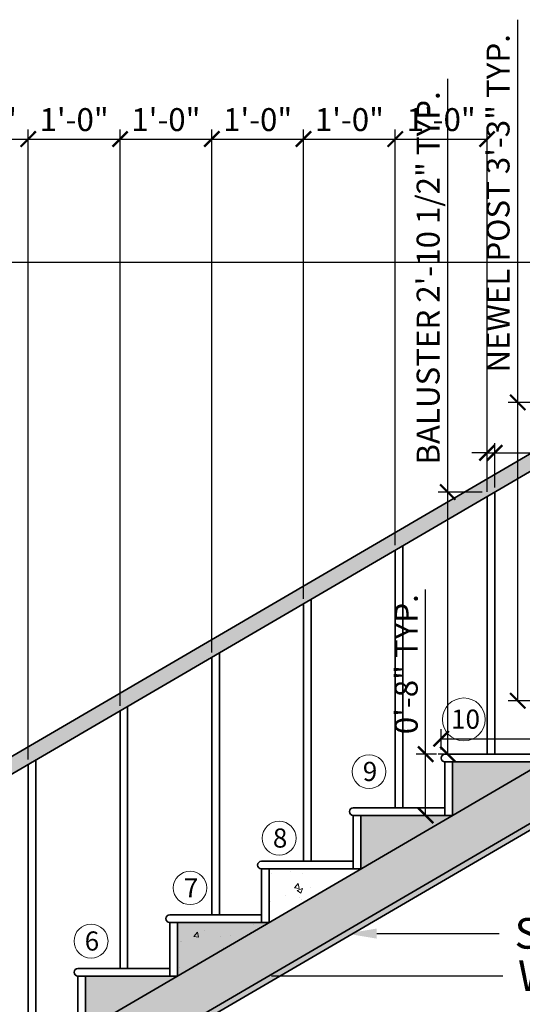
# Model space of a CAD drawing. Units: inches. Extents: x 2205 to 2524, y 4609 to 4803.
# Tile 3 of 5: x 2311 to 2377, y 4674 to 4803. Entities that reach past the tile are written whole.
import ezdxf
from ezdxf import colors
from ezdxf.entities.mleader import LeaderData, LeaderLine
from ezdxf.math import Vec2, Vec3

# ---------------------------------------------------------------- set-up
doc = ezdxf.new("R2010")
doc.units = ezdxf.units.IN
for name, color, linetype, lineweight in [('A-ANNO-DIMS', 2, 'Continuous', 18), ('A-ANNO-SYMB', 3, 'Continuous', 18), ('A-ANNO-TEXT', 7, 'Continuous', 18), ('A-FLOR-STRS', 7, 'Continuous', 35), ('A-SECT-PATT', 252, 'Continuous', 13)]:
    doc.layers.add(name, color=color, linetype=linetype, lineweight=lineweight)
doc.styles.get("Standard").update_dxf_attribs({"font": 'arial.ttf'})
doc.dimstyles.new('ISO-25', dxfattribs={"dimtxt": 3, "dimasz": 2, "dimexe": 1.25, "dimexo": 0.625, "dimtad": 1, "dimdec": 1, "dimlunit": 3, "dimtxsty": 'Standard', "dimblk": 'ARCHTICK', "dimcen": 2.5, "dimclrd": 5, "dimclre": 2, "dimclrt": 6, "dimadec": 0, "dimazin": 0, "dimtfac": 1, "dimtdec": 1, "dimtmove": 0, "dimatfit": 3, "dimfxl": 1, "dimarcsym": 0})

# ---------------------------------------------------------------- blocks, each defined once
blk = doc.blocks.new('STAIR-STEP')
for p, q in [((2282.7, 4650.98), (2270.7, 4650.98)), ((2283.7, 4649.98), (2270.7, 4649.98)), ((2270.7, 4649.98), (2270.7, 4642.98)), ((2271.7, 4649.98), (2271.7, 4642.98))]:
    blk.add_line(p, q)
blk.add_arc((2270.7, 4650.48), 0.5, 90, 270)
blk = doc.blocks.new('BALUSTER')
for p, q in [((2276.2, 4684.66), (2276.2, 4650.98)), ((2277.2, 4685.25), (2277.2, 4650.98))]:
    blk.add_line(p, q)
blk = doc.blocks.new('_ArchTick')
at = {"color": 0, "linetype": 'ByBlock', "const_width": 0.15}
blk.add_lwpolyline([(-0.5, -0.5), (0.5, 0.5)], dxfattribs=at)
blk = doc.blocks.new('*D9')
at = {"layer": 'A-ANNO-DIMS', "color": 2, "lineweight": -2, "transparency": 16777216}
for p, q in [((2366.2, 4707.6), (2366.2, 4710.25)), ((2379.7, 4707.6), (2379.7, 4710.25))]:
    blk.add_line(p, q, dxfattribs=at)
at = {"layer": 'A-ANNO-DIMS', "color": 5, "lineweight": -2, "transparency": 16777216}
for p, q in [((2366.2, 4709), (2379.7, 4709)), ((2379.7, 4709), (2433.83, 4709))]:
    blk.add_line(p, q, dxfattribs=at)
at = {"layer": 'DEFPOINTS', "color": 0, "transparency": 16777216}
for p in [(2379.7, 4709), (2366.2, 4706.98), (2379.7, 4706.98)]:
    blk.add_point(p, dxfattribs=at)
at = {"layer": 'A-ANNO-DIMS', "color": 5, "lineweight": -2, "transparency": 16777216, "xscale": 2, "yscale": 2, "zscale": 2, "rotation": 180}
blk.add_blockref('_ArchTick', (2366.2, 4709), dxfattribs=at)
at = {"layer": 'A-ANNO-DIMS', "color": 5, "lineweight": -2, "transparency": 16777216, "xscale": 2, "yscale": 2, "zscale": 2}
blk.add_blockref('_ArchTick', (2379.7, 4709), dxfattribs=at)
at = {"layer": 'A-ANNO-DIMS', "color": 6, "transparency": 16777216, "insert": (2407.76, 4711.18), "char_height": 3, "attachment_point": 5}
blk.add_mtext('STAIR STEP 1\'-1 1/2" TYP.', dxfattribs=at)
blk = doc.blocks.new('*D10')
at = {"layer": 'A-ANNO-DIMS', "color": 5, "lineweight": -2, "transparency": 16777216}
for p, q in [((2364.17, 4706.98), (2364.17, 4728.52)), ((2364.17, 4698.98), (2364.17, 4706.98))]:
    blk.add_line(p, q, dxfattribs=at)
at = {"layer": 'A-ANNO-DIMS', "color": 2, "lineweight": -2, "transparency": 16777216}
for p, q in [((2365.57, 4706.98), (2362.92, 4706.98)), ((2365.57, 4698.98), (2362.92, 4698.98))]:
    blk.add_line(p, q, dxfattribs=at)
at = {"layer": 'DEFPOINTS', "color": 0, "transparency": 16777216}
for p in [(2364.17, 4706.98), (2366.2, 4706.98), (2366.2, 4698.98)]:
    blk.add_point(p, dxfattribs=at)
at = {"layer": 'A-ANNO-DIMS', "color": 5, "lineweight": -2, "transparency": 16777216, "xscale": 2, "yscale": 2, "zscale": 2}
for p, rotation in [((2364.17, 4706.98), 90), ((2364.17, 4698.98), 270)]:
    blk.add_blockref('_ArchTick', p, dxfattribs=dict(at, rotation=rotation))
at = {"layer": 'A-ANNO-DIMS', "color": 6, "transparency": 16777216, "insert": (2362.02, 4718.75), "char_height": 3, "attachment_point": 5, "rotation": 90}
blk.add_mtext('0\'-8" TYP.', dxfattribs=at)
blk = doc.blocks.new('*D11')
at = {"layer": 'A-ANNO-DIMS', "color": 5, "lineweight": -2, "transparency": 16777216}
for p, q in [((2367.06, 4741.25), (2367.06, 4795.26)), ((2367.06, 4706.98), (2367.06, 4741.25))]:
    blk.add_line(p, q, dxfattribs=at)
at = {"layer": 'A-ANNO-DIMS', "color": 2, "lineweight": -2, "transparency": 16777216}
for p, q in [((2371.57, 4741.25), (2365.81, 4741.25)), ((2371.57, 4706.98), (2365.81, 4706.98))]:
    blk.add_line(p, q, dxfattribs=at)
at = {"layer": 'DEFPOINTS', "color": 0, "transparency": 16777216}
for p in [(2367.06, 4741.25), (2372.2, 4741.25), (2372.2, 4706.98)]:
    blk.add_point(p, dxfattribs=at)
at = {"layer": 'A-ANNO-DIMS', "color": 5, "lineweight": -2, "transparency": 16777216, "xscale": 2, "yscale": 2, "zscale": 2}
for p, rotation in [((2367.06, 4741.25), 90), ((2367.06, 4706.98), 270)]:
    blk.add_blockref('_ArchTick', p, dxfattribs=dict(at, rotation=rotation))
at = {"layer": 'A-ANNO-DIMS', "color": 6, "transparency": 16777216, "insert": (2364.88, 4769.25), "char_height": 3, "attachment_point": 5, "rotation": 90}
blk.add_mtext('BALUSTER 2\'-10 1/2" TYP.', dxfattribs=at)
blk = doc.blocks.new('*D12')
at = {"layer": 'A-ANNO-DIMS', "color": 2, "lineweight": -2, "transparency": 16777216}
for p, q in [((2372.2, 4741.87), (2372.2, 4747.64)), ((2373.2, 4741.87), (2373.2, 4747.64))]:
    blk.add_line(p, q, dxfattribs=at)
at = {"layer": 'A-ANNO-DIMS', "color": 5, "lineweight": -2, "transparency": 16777216}
for p, q in [((2372.2, 4746.39), (2370.2, 4746.39)), ((2372.2, 4746.39), (2373.2, 4746.39)), ((2373.2, 4746.39), (2396.73, 4746.39))]:
    blk.add_line(p, q, dxfattribs=at)
at = {"layer": 'DEFPOINTS', "color": 0, "transparency": 16777216}
for p in [(2373.2, 4746.39), (2372.2, 4741.25), (2373.2, 4741.25)]:
    blk.add_point(p, dxfattribs=at)
at = {"layer": 'A-ANNO-DIMS', "color": 5, "lineweight": -2, "transparency": 16777216, "xscale": 2, "yscale": 2, "zscale": 2}
blk.add_blockref('_ArchTick', (2372.2, 4746.39), dxfattribs=at)
at = {"layer": 'A-ANNO-DIMS', "color": 5, "lineweight": -2, "transparency": 16777216, "xscale": 2, "yscale": 2, "zscale": 2, "rotation": 180}
blk.add_blockref('_ArchTick', (2373.2, 4746.39), dxfattribs=at)
at = {"layer": 'A-ANNO-DIMS', "color": 6, "transparency": 16777216, "insert": (2386.97, 4748.54), "char_height": 3, "attachment_point": 5}
blk.add_mtext('0\'-1" TYP.', dxfattribs=at)
blk = doc.blocks.new('*D13')
at = {"layer": 'A-ANNO-DIMS', "color": 5, "lineweight": -2, "transparency": 16777216}
for p, q in [((2376.21, 4752.98), (2376.21, 4803.01)), ((2376.21, 4713.98), (2376.21, 4752.98))]:
    blk.add_line(p, q, dxfattribs=at)
at = {"layer": 'A-ANNO-DIMS', "color": 2, "lineweight": -2, "transparency": 16777216}
for p, q in [((2381.44, 4752.98), (2374.96, 4752.98)), ((2381.44, 4713.98), (2374.96, 4713.98))]:
    blk.add_line(p, q, dxfattribs=at)
at = {"layer": 'DEFPOINTS', "color": 0, "transparency": 16777216}
for p in [(2376.21, 4752.98), (2382.06, 4752.98), (2382.06, 4713.98)]:
    blk.add_point(p, dxfattribs=at)
at = {"layer": 'A-ANNO-DIMS', "color": 5, "lineweight": -2, "transparency": 16777216, "xscale": 2, "yscale": 2, "zscale": 2}
for p, rotation in [((2376.21, 4752.98), 90), ((2376.21, 4713.98), 270)]:
    blk.add_blockref('_ArchTick', p, dxfattribs=dict(at, rotation=rotation))
at = {"layer": 'A-ANNO-DIMS', "color": 6, "transparency": 16777216, "insert": (2374.03, 4779), "char_height": 3, "attachment_point": 5, "rotation": 90}
blk.add_mtext('NEWEL POST 3\'-3" TYP.', dxfattribs=at)
blk = doc.blocks.new('*D16')
at = {"layer": 'A-ANNO-DIMS', "color": 2, "lineweight": -2, "transparency": 16777216}
for p, q in [((2428.57, 4771.26), (2222.09, 4771.26)), ((2428.57, 4636.98), (2222.09, 4636.98))]:
    blk.add_line(p, q, dxfattribs=at)
at = {"layer": 'A-ANNO-DIMS', "color": 5, "lineweight": -2, "transparency": 16777216}
blk.add_line((2223.34, 4636.98), (2223.34, 4771.26), dxfattribs=at)
at = {"layer": 'DEFPOINTS', "color": 0, "transparency": 16777216}
for p in [(2223.34, 4771.26), (2429.2, 4771.26), (2429.2, 4636.98)]:
    blk.add_point(p, dxfattribs=at)
at = {"layer": 'A-ANNO-DIMS', "color": 5, "lineweight": -2, "transparency": 16777216, "xscale": 2, "yscale": 2, "zscale": 2}
for p, rotation in [((2223.34, 4771.26), 90), ((2223.34, 4636.98), 270)]:
    blk.add_blockref('_ArchTick', p, dxfattribs=dict(at, rotation=rotation))
at = {"layer": 'A-ANNO-DIMS', "color": 6, "transparency": 16777216, "insert": (2221.17, 4704.12), "char_height": 3, "attachment_point": 5, "rotation": 90}
blk.add_mtext('11\'-2 1/2"', dxfattribs=at)
blk = doc.blocks.new('*D29')
at = {"layer": 'A-ANNO-DIMS', "color": 2, "lineweight": -2, "transparency": 16777216}
for p, q in [((2300.2, 4699.29), (2300.2, 4788.66)), ((2312.2, 4706.29), (2312.2, 4788.66))]:
    blk.add_line(p, q, dxfattribs=at)
at = {"layer": 'A-ANNO-DIMS', "color": 5, "lineweight": -2, "transparency": 16777216}
blk.add_line((2300.2, 4787.41), (2312.2, 4787.41), dxfattribs=at)
at = {"layer": 'DEFPOINTS', "color": 0, "transparency": 16777216}
for p in [(2312.2, 4787.41), (2312.2, 4705.66), (2300.2, 4698.66)]:
    blk.add_point(p, dxfattribs=at)
at = {"layer": 'A-ANNO-DIMS', "color": 5, "lineweight": -2, "transparency": 16777216, "xscale": 2, "yscale": 2, "zscale": 2, "rotation": 180}
blk.add_blockref('_ArchTick', (2300.2, 4787.41), dxfattribs=at)
at = {"layer": 'A-ANNO-DIMS', "color": 5, "lineweight": -2, "transparency": 16777216, "xscale": 2, "yscale": 2, "zscale": 2}
blk.add_blockref('_ArchTick', (2312.2, 4787.41), dxfattribs=at)
at = {"layer": 'A-ANNO-DIMS', "color": 6, "transparency": 16777216, "insert": (2306.2, 4789.56), "char_height": 3, "attachment_point": 5}
blk.add_mtext('1\'-0"', dxfattribs=at)
blk = doc.blocks.new('*D30')
at = {"layer": 'A-ANNO-DIMS', "color": 2, "lineweight": -2, "transparency": 16777216}
for p, q in [((2312.2, 4706.29), (2312.2, 4788.66)), ((2324.2, 4713.29), (2324.2, 4788.66))]:
    blk.add_line(p, q, dxfattribs=at)
at = {"layer": 'A-ANNO-DIMS', "color": 5, "lineweight": -2, "transparency": 16777216}
blk.add_line((2312.2, 4787.41), (2324.2, 4787.41), dxfattribs=at)
at = {"layer": 'DEFPOINTS', "color": 0, "transparency": 16777216}
for p in [(2324.2, 4787.41), (2324.2, 4712.66), (2312.2, 4705.66)]:
    blk.add_point(p, dxfattribs=at)
at = {"layer": 'A-ANNO-DIMS', "color": 5, "lineweight": -2, "transparency": 16777216, "xscale": 2, "yscale": 2, "zscale": 2, "rotation": 180}
blk.add_blockref('_ArchTick', (2312.2, 4787.41), dxfattribs=at)
at = {"layer": 'A-ANNO-DIMS', "color": 5, "lineweight": -2, "transparency": 16777216, "xscale": 2, "yscale": 2, "zscale": 2}
blk.add_blockref('_ArchTick', (2324.2, 4787.41), dxfattribs=at)
at = {"layer": 'A-ANNO-DIMS', "color": 6, "transparency": 16777216, "insert": (2318.2, 4789.56), "char_height": 3, "attachment_point": 5}
blk.add_mtext('1\'-0"', dxfattribs=at)
blk = doc.blocks.new('*D31')
at = {"layer": 'A-ANNO-DIMS', "color": 2, "lineweight": -2, "transparency": 16777216}
for p, q in [((2324.2, 4713.29), (2324.2, 4788.66)), ((2336.2, 4720.29), (2336.2, 4788.66))]:
    blk.add_line(p, q, dxfattribs=at)
at = {"layer": 'A-ANNO-DIMS', "color": 5, "lineweight": -2, "transparency": 16777216}
blk.add_line((2324.2, 4787.41), (2336.2, 4787.41), dxfattribs=at)
at = {"layer": 'DEFPOINTS', "color": 0, "transparency": 16777216}
for p in [(2336.2, 4787.41), (2336.2, 4719.66), (2324.2, 4712.66)]:
    blk.add_point(p, dxfattribs=at)
at = {"layer": 'A-ANNO-DIMS', "color": 5, "lineweight": -2, "transparency": 16777216, "xscale": 2, "yscale": 2, "zscale": 2, "rotation": 180}
blk.add_blockref('_ArchTick', (2324.2, 4787.41), dxfattribs=at)
at = {"layer": 'A-ANNO-DIMS', "color": 5, "lineweight": -2, "transparency": 16777216, "xscale": 2, "yscale": 2, "zscale": 2}
blk.add_blockref('_ArchTick', (2336.2, 4787.41), dxfattribs=at)
at = {"layer": 'A-ANNO-DIMS', "color": 6, "transparency": 16777216, "insert": (2330.2, 4789.56), "char_height": 3, "attachment_point": 5}
blk.add_mtext('1\'-0"', dxfattribs=at)
blk = doc.blocks.new('*D32')
at = {"layer": 'A-ANNO-DIMS', "color": 2, "lineweight": -2, "transparency": 16777216}
for p, q in [((2336.2, 4720.29), (2336.2, 4788.66)), ((2348.2, 4727.29), (2348.2, 4788.66))]:
    blk.add_line(p, q, dxfattribs=at)
at = {"layer": 'A-ANNO-DIMS', "color": 5, "lineweight": -2, "transparency": 16777216}
blk.add_line((2336.2, 4787.41), (2348.2, 4787.41), dxfattribs=at)
at = {"layer": 'DEFPOINTS', "color": 0, "transparency": 16777216}
for p in [(2348.2, 4787.41), (2348.2, 4726.66), (2336.2, 4719.66)]:
    blk.add_point(p, dxfattribs=at)
at = {"layer": 'A-ANNO-DIMS', "color": 5, "lineweight": -2, "transparency": 16777216, "xscale": 2, "yscale": 2, "zscale": 2, "rotation": 180}
blk.add_blockref('_ArchTick', (2336.2, 4787.41), dxfattribs=at)
at = {"layer": 'A-ANNO-DIMS', "color": 5, "lineweight": -2, "transparency": 16777216, "xscale": 2, "yscale": 2, "zscale": 2}
blk.add_blockref('_ArchTick', (2348.2, 4787.41), dxfattribs=at)
at = {"layer": 'A-ANNO-DIMS', "color": 6, "transparency": 16777216, "insert": (2342.2, 4789.56), "char_height": 3, "attachment_point": 5}
blk.add_mtext('1\'-0"', dxfattribs=at)
blk = doc.blocks.new('*D33')
at = {"layer": 'A-ANNO-DIMS', "color": 2, "lineweight": -2, "transparency": 16777216}
for p, q in [((2348.2, 4727.29), (2348.2, 4788.66)), ((2360.2, 4734.29), (2360.2, 4788.66))]:
    blk.add_line(p, q, dxfattribs=at)
at = {"layer": 'A-ANNO-DIMS', "color": 5, "lineweight": -2, "transparency": 16777216}
blk.add_line((2348.2, 4787.41), (2360.2, 4787.41), dxfattribs=at)
at = {"layer": 'DEFPOINTS', "color": 0, "transparency": 16777216}
for p in [(2360.2, 4787.41), (2360.2, 4733.66), (2348.2, 4726.66)]:
    blk.add_point(p, dxfattribs=at)
at = {"layer": 'A-ANNO-DIMS', "color": 5, "lineweight": -2, "transparency": 16777216, "xscale": 2, "yscale": 2, "zscale": 2, "rotation": 180}
blk.add_blockref('_ArchTick', (2348.2, 4787.41), dxfattribs=at)
at = {"layer": 'A-ANNO-DIMS', "color": 5, "lineweight": -2, "transparency": 16777216, "xscale": 2, "yscale": 2, "zscale": 2}
blk.add_blockref('_ArchTick', (2360.2, 4787.41), dxfattribs=at)
at = {"layer": 'A-ANNO-DIMS', "color": 6, "transparency": 16777216, "insert": (2354.2, 4789.56), "char_height": 3, "attachment_point": 5}
blk.add_mtext('1\'-0"', dxfattribs=at)
blk = doc.blocks.new('*D34')
at = {"layer": 'A-ANNO-DIMS', "color": 2, "lineweight": -2, "transparency": 16777216}
for p, q in [((2360.2, 4734.29), (2360.2, 4788.66)), ((2372.2, 4741.29), (2372.2, 4788.66))]:
    blk.add_line(p, q, dxfattribs=at)
at = {"layer": 'A-ANNO-DIMS', "color": 5, "lineweight": -2, "transparency": 16777216}
blk.add_line((2360.2, 4787.41), (2372.2, 4787.41), dxfattribs=at)
at = {"layer": 'DEFPOINTS', "color": 0, "transparency": 16777216}
for p in [(2372.2, 4787.41), (2372.2, 4740.66), (2360.2, 4733.66)]:
    blk.add_point(p, dxfattribs=at)
at = {"layer": 'A-ANNO-DIMS', "color": 5, "lineweight": -2, "transparency": 16777216, "xscale": 2, "yscale": 2, "zscale": 2, "rotation": 180}
blk.add_blockref('_ArchTick', (2360.2, 4787.41), dxfattribs=at)
at = {"layer": 'A-ANNO-DIMS', "color": 5, "lineweight": -2, "transparency": 16777216, "xscale": 2, "yscale": 2, "zscale": 2}
blk.add_blockref('_ArchTick', (2372.2, 4787.41), dxfattribs=at)
at = {"layer": 'A-ANNO-DIMS', "color": 6, "transparency": 16777216, "insert": (2366.2, 4789.56), "char_height": 3, "attachment_point": 5}
blk.add_mtext('1\'-0"', dxfattribs=at)

msp = doc.modelspace()

# ---------------------------------------------------------------- hatches: boundary and pattern name
at = {"layer": 'A-SECT-PATT'}
h = msp.add_hatch(dxfattribs=at)
h.set_pattern_fill('AR-CONC', color=256, scale=0.04)
h.paths.add_polyline_path([(2393.32, 4706.98), (2419.45, 4706.98), (2425.45, 4706.98), (2425.45, 4712.98), (2419.45, 4712.98), (2379.7, 4712.98), (2379.7, 4705.98), (2271.7, 4642.98), (2259.7, 4636.98), (2273.32, 4636.98)])
h.paths.add_polyline_path([(2343.7, 4684.98), (2331.7, 4684.98), (2331.7, 4677.98)], flags=16)
h.paths.add_polyline_path([(2331.7, 4677.98), (2319.7, 4677.98), (2319.7, 4670.98)], flags=16)
h.paths.add_polyline_path([(2319.7, 4670.98), (2307.7, 4670.98), (2307.7, 4663.98)], flags=16)
h.paths.add_polyline_path([(2307.7, 4663.98), (2295.7, 4663.98), (2295.7, 4656.98)], flags=16)
h.paths.add_polyline_path([(2295.7, 4656.98), (2283.7, 4656.98), (2283.7, 4649.98)], flags=16)
h.paths.add_polyline_path([(2283.7, 4649.98), (2271.7, 4649.98), (2271.7, 4642.98)], flags=17)
h.paths.add_polyline_path([(2271.7, 4642.98), (2259.7, 4642.98), (2259.7, 4636.98)], flags=17)
h.paths.add_polyline_path([(2379.7, 4705.98), (2367.7, 4705.98), (2367.7, 4698.98)], flags=16)
h.paths.add_polyline_path([(2367.7, 4698.98), (2355.7, 4698.98), (2355.7, 4691.98)], flags=16)
h.paths.add_polyline_path([(2419.45, 4706.98), (2393.32, 4706.98), (2273.32, 4636.98), (2274.81, 4636.98), (2393.52, 4706.23), (2419.45, 4706.23)], flags=17)
h.paths.add_polyline_path([(2419.45, 4706.23), (2418.7, 4706.23), (2418.7, 4636.98), (2419.45, 4636.98)], flags=16)
h.paths.add_polyline_path([(2429.2, 4771.26), (2428.45, 4771.26), (2428.45, 4636.98), (2429.2, 4636.98)])
h.paths.add_polyline_path([(2419.45, 4771.26), (2418.7, 4771.26), (2418.7, 4713.98), (2419.45, 4713.98)])
h = msp.add_hatch(color=256, dxfattribs=at)
h.dxf.hatch_style = 1
h.paths.add_polyline_path([(2264.7, 4678.86, -0.206977), (2261.7, 4678.86), (2261.7, 4643.98), (2264.7, 4643.98)])
h.paths.add_polyline_path([(2261.7, 4681.48, 1), (2264.7, 4681.48, 1)])
h.paths.add_polyline_path([(2382.06, 4746.42), (2382.06, 4748.73), (2264.2, 4679.98), (2264.69, 4679.98), (2264.7, 4679.98), (2264.7, 4677.96)])
h.paths.add_polyline_path([(2418.7, 4748.73), (2385.06, 4748.73), (2385.06, 4746.73), (2418.7, 4746.73)])
h.paths.add_polyline_path([(2385.06, 4748.86, -0.206977), (2382.06, 4748.86), (2382.06, 4713.98), (2385.06, 4713.98)])
h.paths.add_polyline_path([(2382.06, 4751.48, 1), (2385.06, 4751.48, 1)])
h = msp.add_hatch(dxfattribs=at)
h.set_pattern_fill('AR-CONC', color=256, scale=0.04)
h.paths.add_polyline_path([(2355.7, 4691.98), (2343.7, 4691.98), (2343.7, 4684.98)])
h.paths.add_polyline_path([(2343.7, 4684.98), (2331.7, 4684.98), (2331.7, 4677.98)])

# ---------------------------------------------------------------- linework, layer by layer
at = {"layer": 'A-ANNO-SYMB'}
for centre, radius in [((2369.16, 4711.53), 2.8), ((2356.77, 4704.7), 2.21), ((2345.01, 4696), 2.22), ((2333.36, 4689.5), 2.19), ((2320.41, 4682.54), 2.22)]:
    msp.add_circle(centre, radius, dxfattribs=at)
at = {"layer": 'A-FLOR-STRS'}
for p, q in [((2264.2, 4679.98), (2382.06, 4748.73)), ((2264.7, 4677.96), (2382.06, 4746.42)), ((2273.32, 4636.98), (2393.32, 4706.98)), ((2271.7, 4642.98), (2379.7, 4705.98)), ((2274.81, 4636.98), (2393.52, 4706.23))]:
    msp.add_line(p, q, dxfattribs=at)

# ---------------------------------------------------------------- block references
for name, p in [('BALUSTER', (96, 56)), ('BALUSTER', (84, 49)), ('BALUSTER', (72, 42)), ('BALUSTER', (60, 35)), ('BALUSTER', (48, 28)), ('STAIR-STEP', (96, 56)), ('BALUSTER', (36, 21)), ('STAIR-STEP', (84, 49)), ('STAIR-STEP', (72, 42)), ('STAIR-STEP', (60, 35)), ('STAIR-STEP', (48, 28))]:
    msp.add_blockref(name, p, dxfattribs=at)

# ---------------------------------------------------------------- texts
at = {"layer": 'A-ANNO-TEXT', "char_height": 2.5, "attachment_point": 1}
for s, insert in [('10', (2367.49, 4712.81)), ('9', (2355.95, 4705.98)), ('8', (2344.19, 4697.27)), ('7', (2332.55, 4690.75)), ('6', (2319.58, 4683.81))]:
    msp.add_mtext_dynamic_manual_height_columns(s, width=3.6522, gutter_width=12.5, heights=[0], dxfattribs=dict(at, insert=insert))

# ---------------------------------------------------------------- dimensions: what is measured, and where the dimension line sits
at = {"layer": 'A-ANNO-DIMS'}
for base, p1, p2, text, picture, middle in [((2376.21, 4752.98), (2382.06, 4713.98), (2382.06, 4752.98), 'NEWEL POST <> TYP.', '*D13', (2374.03, 4779)), ((2367.06, 4741.25), (2372.2, 4706.98), (2372.2, 4741.25), 'BALUSTER <> TYP.', '*D11', (2364.88, 4769.25)), ((2364.17, 4706.98), (2366.2, 4698.98), (2366.2, 4706.98), '<> TYP.', '*D10', (2362.02, 4718.75))]:
    dim = msp.add_linear_dim(base=base, p1=p1, p2=p2, angle=90, text=text, dimstyle='ISO-25', override={"dimdec": 1, "dimrnd": 0, "dimzin": 1, "dimlunit": 4, "dimfrac": 2}, dxfattribs=at)
    dim.commit()
    dim.dimension.update_dxf_attribs({"geometry": picture, "text_midpoint": middle})
for base, p1, p2, picture, middle in [((2312.2, 4787.41), (2300.2, 4698.66), (2312.2, 4705.66), '*D29', (2306.2, 4789.56)), ((2324.2, 4787.41), (2312.2, 4705.66), (2324.2, 4712.66), '*D30', (2318.2, 4789.56)), ((2336.2, 4787.41), (2324.2, 4712.66), (2336.2, 4719.66), '*D31', (2330.2, 4789.56)), ((2348.2, 4787.41), (2336.2, 4719.66), (2348.2, 4726.66), '*D32', (2342.2, 4789.56)), ((2360.2, 4787.41), (2348.2, 4726.66), (2360.2, 4733.66), '*D33', (2354.2, 4789.56)), ((2372.2, 4787.41), (2360.2, 4733.66), (2372.2, 4740.66), '*D34', (2366.2, 4789.56))]:
    dim = msp.add_linear_dim(base=base, p1=p1, p2=p2, dimstyle='ISO-25', override={"dimdec": 1, "dimlfac": 1, "dimrnd": 0, "dimzin": 1, "dimdsep": 46, "dimlunit": 4, "dimfrac": 2}, dxfattribs=at)
    dim.commit()
    dim.dimension.update_dxf_attribs({"geometry": picture, "text_midpoint": middle})
dim = msp.add_linear_dim(base=(2223.34, 4771.26), p1=(2429.2, 4636.98), p2=(2429.2, 4771.26), angle=90, dimstyle='ISO-25', override={"dimdec": 1, "dimlfac": 1, "dimrnd": 0, "dimzin": 1, "dimdsep": 46, "dimlunit": 4, "dimfrac": 2}, dxfattribs=at)
dim.commit()
dim.dimension.update_dxf_attribs({"geometry": '*D16', "text_midpoint": (2221.17, 4704.12)})
for base, p1, p2, text, picture, middle in [((2373.2, 4746.39), (2372.2, 4741.25), (2373.2, 4741.25), '<> TYP.', '*D12', (2386.97, 4748.54)), ((2379.7, 4709), (2366.2, 4706.98), (2379.7, 4706.98), 'STAIR STEP <> TYP.', '*D9', (2407.76, 4711.18))]:
    dim = msp.add_linear_dim(base=base, p1=p1, p2=p2, text=text, dimstyle='ISO-25', override={"dimdec": 1, "dimrnd": 0, "dimzin": 1, "dimlunit": 4, "dimfrac": 2}, dxfattribs=at)
    dim.commit()
    dim.dimension.update_dxf_attribs({"geometry": picture, "text_midpoint": middle})

# ---------------------------------------------------------------- leaders
at = {"layer": 'A-ANNO-SYMB'}
ml = msp.add_multileader_mtext('Standard', dxfattribs=at)
ml.set_content('SOFFIT', color=256)
ml.set_leader_properties()
ml.build(insert=Vec2(0, 0))
ctx = ml.context
ctx.base_point, ctx.plane_origin = Vec3(2373.8, 4683.53), Vec3(2353.78, 4683.53)
notes = []
notes.append((ctx, [(0, (1, 1, 0), (2365.8, 4683.53), (1, 0), 8, [(0, [(2353.78, 4683.53)], 0, [])])]))
ctx.mtext.insert, ctx.mtext.width, ctx.mtext.flow_direction = Vec3(2375.8, 4685.56), 53.5271, 5
ml = msp.add_multileader_mtext('Standard', dxfattribs=at)
ml.set_content('WAIST', color=256)
ml.set_leader_properties()
ml.build(insert=Vec2(0, 0))
ctx = ml.context
ctx.base_point, ctx.plane_origin = Vec3(2374.25, 4677.99), Vec3(2340.01, 4677.99)
notes.append((ctx, [(0, (1, 1, 0), (2352.03, 4677.99), (1, 0), 22.22, [(0, [(2340.01, 4677.99)], 0, [])])]))
ctx.mtext.insert, ctx.mtext.width, ctx.mtext.flow_direction = Vec3(2376.25, 4680.02), 53.5271, 5
for ctx, leaders in notes:
    for number, flags, end, landing, length, lines in leaders:
        leader = LeaderData()
        leader.index, (leader.has_last_leader_line, leader.has_dogleg_vector, leader.attachment_direction) = number, flags
        leader.last_leader_point, leader.dogleg_vector, leader.dogleg_length = Vec3(end), Vec3(landing), length
        for number, points, colour, breaks in lines:
            line = LeaderLine()
            line.index, line.vertices, line.color, line.breaks = number, Vec3.list(points), colors.encode_raw_color(colour), breaks
            leader.lines.append(line)
        ctx.leaders.append(leader)

doc.saveas('drawing.dxf')
